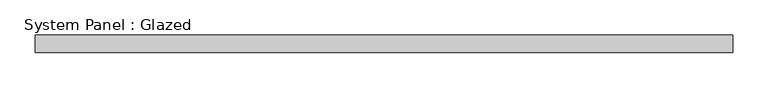
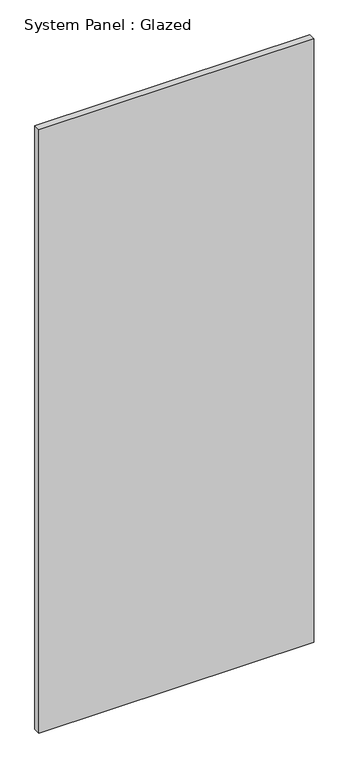
"""IFC4 building model written with IfcOpenShell, lengths in millimetres: plate geometry, System Panel : Glazed."""

from ifc_helpers import new_model, si_unit, origin, origin_with_axes, place, context, project, spatial, polyline, outline, extrude, source, transform, mapped, element, save


def system_panel_glazed_7ebbbc7e(model_context):
    return source(origin(), model_context, "Body", "SweptSolid", [
        extrude(outline(polyline([(498.4750001, 19.05), (-498.4750001, 19.05), (-498.4750001, 44.45), (498.4750001, 44.45), (498.4750001, 19.05)])), origin_with_axes(), (0.0, 0.0, 1.0), 2311.4),
    ])


if __name__ == "__main__":
    model = new_model("IFC4")
    model_context = context("Model", 3, world=origin())
    ifc_project = project(units=[si_unit("LENGTHUNIT", "METRE", prefix="MILLI")], contexts=[model_context])
    site = spatial("IfcSite", under=ifc_project)
    building = spatial("IfcBuilding", under=site)
    placement = place(None, origin())
    system_panel_glazed_shape = system_panel_glazed_7ebbbc7e(model_context)
    element("IfcPlate", 1, ObjectType="System Panel : Glazed", at=placement, inside=building, context=model_context, shape_type="MappedRepresentation", body=[
        mapped(system_panel_glazed_shape, transform((0.0, 0.0, 0.0), x_axis=(1.0, 0.0, 0.0), y_axis=(0.0, 1.0, 0.0), z_axis=(0.0, 0.0, 1.0))),
    ])
    save(model, "model.ifc")

# Revit data of these elements
# Type "System Panel : Glazed"
#   Construction Type Id = "GSP4R"
#   Analytic Construction = "1/8 in Pilkington single glazing"
#   Visual Light Transmittance = 0.9
#   Solar Heat Gain Coefficient = 0.86
#   Heat Transfer Coefficient (U) = 1.18115 BTU/(h·ft²·°F)
#   Define Thermal Properties by = 1
# Element 1 (IfcPlate, "System Panel : Glazed")
#   Materials on its faces: "Glass"
# Materials
#   "Glass": class "Glass", colour RGB 0 128 192, transparency 0.75, Description = "Soda Lime Glass", Cost = 0
